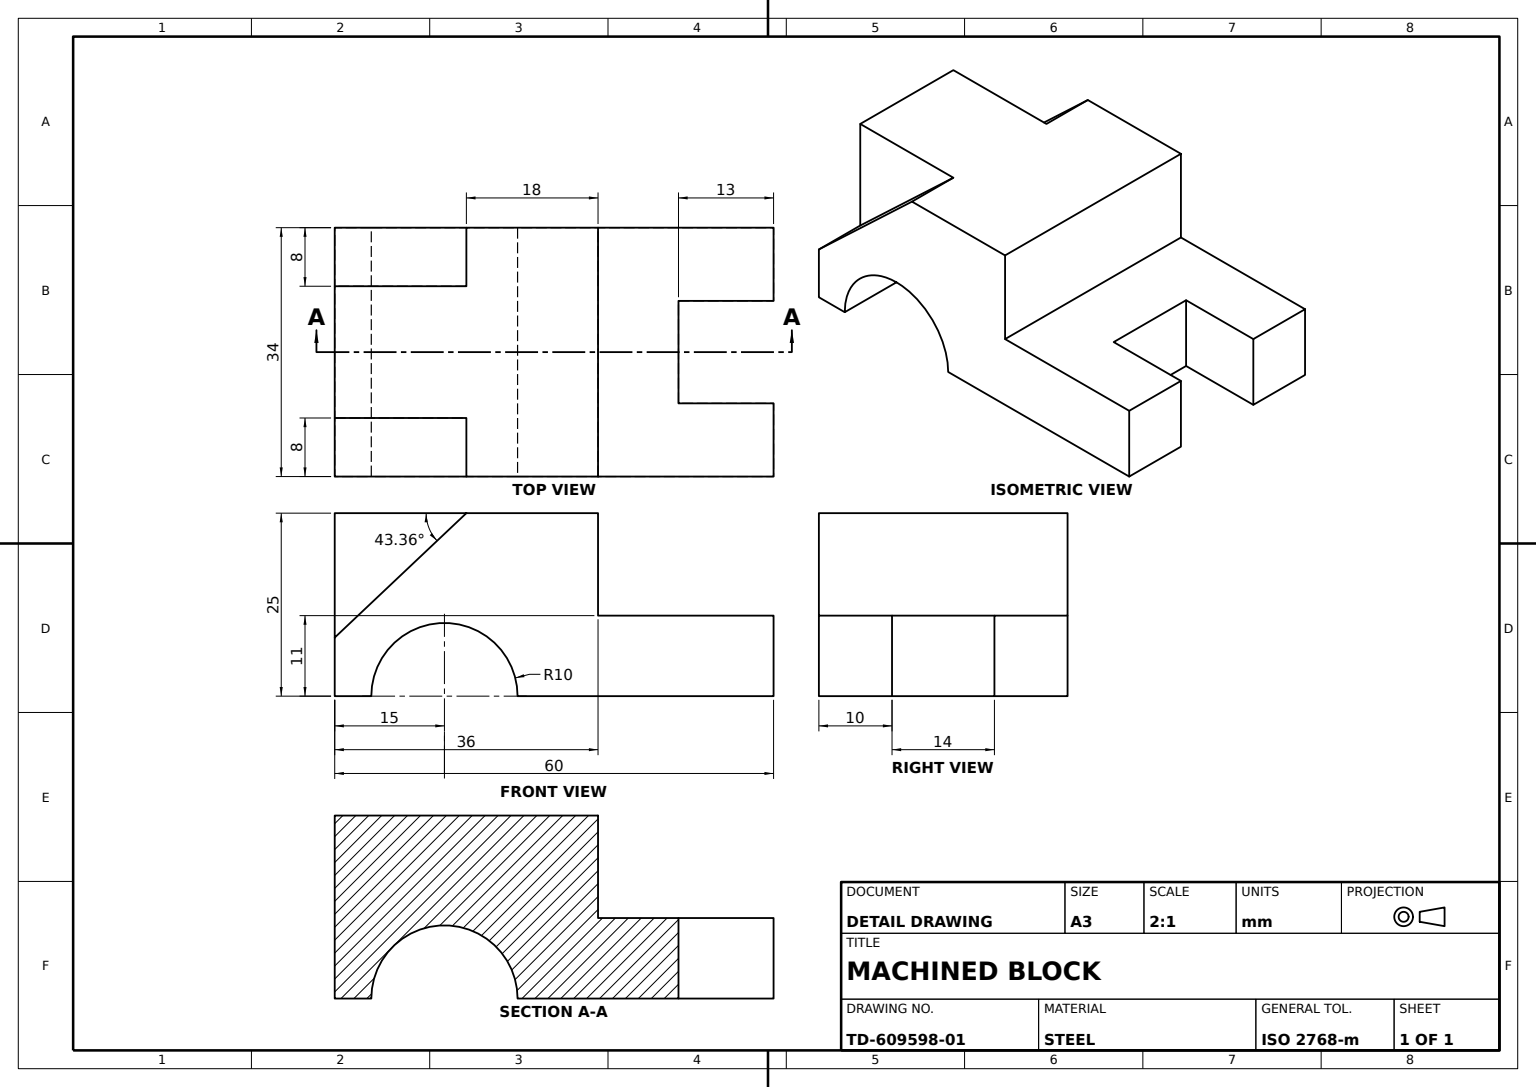
SolidWorks part; units mm, degrees
material "Plain Carbon Steel"
ref_plane "Front Plane" through (0, 0, 0) normal (0, 0, 1) x (1, 0, 0)
ref_plane "Top Plane" through (0, 0, 0) normal (0, 1, 0) x (1, 0, 0)
ref_plane "Right Plane" through (0, 0, 0) normal (1, 0, 0) x (0, 0, -1)
sketch "Base Block Profile" plane through (0, 0, 0) normal (0, 0, 1) x (1, 0, 0)
  line L0 (-15, 0) -> (-15, 25)
  line L1 (-15, 25) -> (21, 25)
  line L2 (21, 25) -> (21, 11)
  line L3 (21, 11) -> (45, 11)
  line L4 (45, 11) -> (45, 0)
  line L5 (45, 0) -> (10, 0)
  line L6 (-10, 0) -> (-15, 0)
  arc A0 (10, 0) -> (-10, 0) centre (0, 0) ccw
  dimension "D4" = 10
  dimension "D1" = 36
  dimension "D2" = 25
  dimension "D3" = 11
  dimension "D5" = 60
  dimension "D6" = 15
extrude "Base Block" add sketch "Base Block Profile" along normal mid plane 34
sketch "End Slot Sketch" plane through (0, 11, 0) normal (0, 1, 0) x (1, 0, 0)
  line L0 (45, 7) -> (32, 7)
  line L1 (45, -17) -> (45, 17) construction
  line L2 (32, 7) -> (32, -7)
  line L3 (32, -7) -> (45, -7)
  line L4 (45, -7) -> (45, 7)
  line L6 (45, 17) -> (21, 17) construction
  dimension "D1" = 13
  dimension "D2" = 14
  dimension "D3" = 10
extrude "End Slot 14x13" cut sketch "End Slot Sketch" against normal mid plane 34
sketch "Half-Round Notch Sketch" plane through (0, 0, 17) normal (0, 0, 1) x (1, 0, 0)
  line L0 (-15, 0) -> (-15, 8) construction
  line L1 (-15, 25) -> (-15, 0) construction
  line L2 (-15, 8) -> (3, 25)
  line L3 (21, 25) -> (-15, 25) construction
  dimension "D1" = 8
extrude "Half-Round Notch R8" cut sketch "Half-Round Notch Sketch" against normal blind 8 and the other way through all
sketch "Side Profile Cut Sketch" plane through (0, 0, -17) normal (0, 0, -1) x (-1, 0, 0)
  line L3 (-3, 25) -> (15, 8)
  line L4 (15, 25) -> (-3, 25)
  line L5 (15, 8) -> (15, 25)
  line L6 (-3, 25) -> (15, 8)
  line L7 (10, 0) -> (15, 0)
  line L8 (15, 0) -> (15, 25)
  line L9 (15, 25) -> (-21, 25)
  line L10 (-21, 25) -> (-21, 11)
  line L11 (-21, 11) -> (-45, 11)
  line L12 (-45, 11) -> (-45, 0)
  line L13 (-45, 0) -> (-10, 0)
  line L14 (10, 0) -> (15, 0)
  line L15 (15, 0) -> (15, 25)
  line L16 (15, 25) -> (-21, 25)
  line L17 (-21, 25) -> (-21, 11)
  line L18 (-21, 11) -> (-45, 11)
  line L19 (-45, 11) -> (-45, 0)
  line L20 (-45, 0) -> (-10, 0)
  line L21 (15, 25) -> (-3, 25)
  line L22 (15, 8) -> (15, 25)
  arc A1 (10, 0) -> (-10, 0) centre (0, 0) ccw
  arc A2 (10, 0) -> (-10, 0) centre (0, 0) ccw
  line M13 (15, 0) -> (15, 25)
  line M14 (15, 25) -> (-21, 25)
  dimension "D1" = 0
  dimension "D2" = 0
extrude "Side Profile Cut" cut sketch "Side Profile Cut Sketch" against normal blind 8 contours L6 M14 M13
